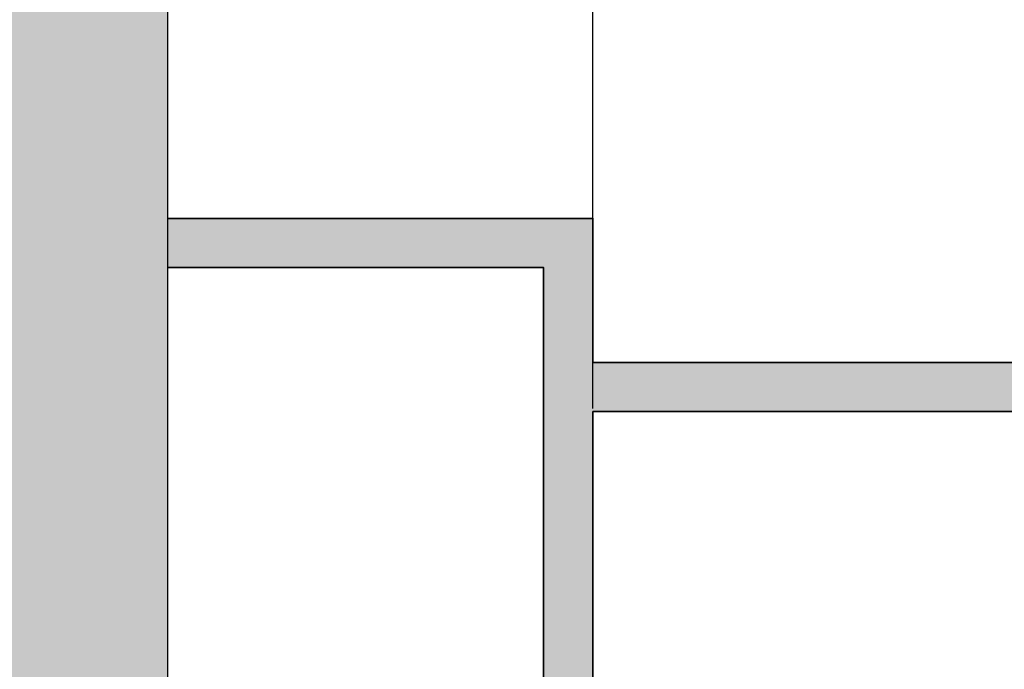
# Model space of a CAD drawing. Units: millimetres. Extents: x -22994 to 29398, y -19990 to 20176.
# Tile 29 of 135: x 99 to 119, y 43 to 56. Entities that reach past the tile are written whole.
import ezdxf

# ---------------------------------------------------------------- set-up
doc = ezdxf.new("R2010")
doc.units = ezdxf.units.MM
doc.header["$MEASUREMENT"] = 0
for name, color, linetype, lineweight in [('M-DIMS', 2, 'Continuous', 18), ('M-EQPM', 7, 'Continuous', 25), ('M-EQPM-PATT', 7, 'Continuous', 18), ('M-PIPE', 7, 'Continuous', 35)]:
    doc.layers.add(name, color=color, linetype=linetype, lineweight=lineweight)
doc.styles.get("Standard").update_dxf_attribs({"font": 'arial.ttf'})
doc.dimstyles.get("Standard").update_dxf_attribs({"dimtxt": 0.18, "dimasz": 10000, "dimexe": 0.18, "dimexo": 0.0625, "dimgap": 0.09, "dimtad": 0, "dimtih": 1, "dimtoh": 1, "dimdec": 0, "dimzin": 0, "dimdsep": 46, "dimtxsty": 'Standard', "dimcen": 0.09, "dimadec": 0, "dimazin": 0, "dimtfac": 1, "dimtdec": 0, "dimtofl": 0, "dimtmove": 0, "dimatfit": 3, "dimfxl": 1, "dimtolj": 1, "dimtzin": 0, "dimlwd": 30, "dimarcsym": 0})

# ---------------------------------------------------------------- blocks, each defined once
blk = doc.blocks.new('*D2')
at = {"layer": 'Defpoints', "color": 0, "transparency": 16777216}
for p in [(6.677, 10.271), (290.852, 10.271), (290.852, -5.079)]:
    blk.add_point(p, dxfattribs=at)
at = {"layer": 'M-DIMS', "color": 0, "lineweight": -2, "transparency": 16777216}
for p, q in [((6.677, 10.209), (6.677, -5.259)), ((290.852, 10.209), (290.852, -5.259))]:
    blk.add_line(p, q, dxfattribs=at)
at = {"layer": 'M-DIMS', "color": 0, "lineweight": 30, "transparency": 16777216}
for p, q in [((-9993.323, -5.079), (-19993.323, -5.079)), ((10290.852, -5.079), (20290.852, -5.079))]:
    blk.add_line(p, q, dxfattribs=at)
at = {"layer": 'M-DIMS', "color": 0, "transparency": 16777216}
for points in [[(-9993.323, 1661.588), (-9993.323, -1671.745), (6.677, -5.079)], [(10290.852, 1661.588), (10290.852, -1671.745), (290.852, -5.079)]]:
    blk.add_solid(points, dxfattribs=at)
at = {"layer": 'M-DIMS', "color": 0, "transparency": 16777216, "insert": (148.765, -5.079), "char_height": 0.18, "attachment_point": 5}
blk.add_mtext('\\A1;284.2', dxfattribs=at)
blk = doc.blocks.new('*D3')
at = {"layer": 'Defpoints', "color": 0, "transparency": 16777216}
for p in [(110.265, 204.165), (110.265, 176.366), (95.833, 127.967)]:
    blk.add_point(p, dxfattribs=at)
at = {"layer": 'M-DIMS', "color": 0, "lineweight": -2, "transparency": 16777216}
for p, q in [((95.833, 128.03), (95.833, 204.345)), ((110.265, 176.429), (110.265, 204.345))]:
    blk.add_line(p, q, dxfattribs=at)
at = {"layer": 'M-DIMS', "color": 0, "lineweight": 30, "transparency": 16777216}
for p, q in [((-9904.167, 204.165), (-19904.167, 204.165)), ((10110.265, 204.165), (20110.265, 204.165))]:
    blk.add_line(p, q, dxfattribs=at)
at = {"layer": 'M-DIMS', "color": 0, "transparency": 16777216}
for points in [[(-9904.167, 1870.832), (-9904.167, -1462.501), (95.833, 204.165)], [(10110.265, 1870.832), (10110.265, -1462.501), (110.265, 204.165)]]:
    blk.add_solid(points, dxfattribs=at)
at = {"layer": 'M-DIMS', "color": 0, "transparency": 16777216, "insert": (103.049, 204.165), "char_height": 0.18, "attachment_point": 5}
blk.add_mtext('\\A1;14.432', dxfattribs=at)
blk = doc.blocks.new('*D4')
at = {"layer": 'Defpoints', "color": 0, "transparency": 16777216}
for p in [(116.265, 204.165), (110.265, 176.366), (116.265, 176.366)]:
    blk.add_point(p, dxfattribs=at)
at = {"layer": 'M-DIMS', "color": 0, "lineweight": -2, "transparency": 16777216}
for p, q in [((110.265, 176.429), (110.265, 204.345)), ((116.265, 176.429), (116.265, 204.345))]:
    blk.add_line(p, q, dxfattribs=at)
at = {"layer": 'M-DIMS', "color": 0, "lineweight": 30, "transparency": 16777216}
for p, q in [((-9889.735, 204.165), (-19889.735, 204.165)), ((10116.265, 204.165), (20116.265, 204.165))]:
    blk.add_line(p, q, dxfattribs=at)
at = {"layer": 'M-DIMS', "color": 0, "transparency": 16777216}
for points in [[(-9889.735, 1870.832), (-9889.735, -1462.501), (110.265, 204.165)], [(10116.265, 1870.832), (10116.265, -1462.501), (116.265, 204.165)]]:
    blk.add_solid(points, dxfattribs=at)
at = {"layer": 'M-DIMS', "color": 0, "transparency": 16777216, "insert": (113.265, 204.165), "char_height": 0.18, "attachment_point": 5}
blk.add_mtext('\\A1;6', dxfattribs=at)
blk = doc.blocks.new('*D5')
at = {"layer": 'Defpoints', "color": 0, "transparency": 16777216}
for p in [(181.265, 204.165), (116.265, 176.366), (181.265, 176.366)]:
    blk.add_point(p, dxfattribs=at)
at = {"layer": 'M-DIMS', "color": 0, "lineweight": -2, "transparency": 16777216}
for p, q in [((116.265, 176.429), (116.265, 204.345)), ((181.265, 176.429), (181.265, 204.345))]:
    blk.add_line(p, q, dxfattribs=at)
at = {"layer": 'M-DIMS', "color": 0, "lineweight": 30, "transparency": 16777216}
for p, q in [((-9883.735, 204.165), (-19883.735, 204.165)), ((10181.265, 204.165), (20181.265, 204.165))]:
    blk.add_line(p, q, dxfattribs=at)
at = {"layer": 'M-DIMS', "color": 0, "transparency": 16777216}
for points in [[(-9883.735, 1870.832), (-9883.735, -1462.501), (116.265, 204.165)], [(10181.265, 1870.832), (10181.265, -1462.501), (181.265, 204.165)]]:
    blk.add_solid(points, dxfattribs=at)
at = {"layer": 'M-DIMS', "color": 0, "transparency": 16777216, "insert": (148.765, 204.165), "char_height": 0.18, "attachment_point": 5}
blk.add_mtext('\\A1;65', dxfattribs=at)
blk = doc.blocks.new('*D6')
at = {"layer": 'Defpoints', "color": 0, "transparency": 16777216}
for p in [(187.265, 204.165), (181.265, 176.366), (187.265, 176.366)]:
    blk.add_point(p, dxfattribs=at)
at = {"layer": 'M-DIMS', "color": 0, "lineweight": -2, "transparency": 16777216}
for p, q in [((181.265, 176.429), (181.265, 204.345)), ((187.265, 176.429), (187.265, 204.345))]:
    blk.add_line(p, q, dxfattribs=at)
at = {"layer": 'M-DIMS', "color": 0, "lineweight": 30, "transparency": 16777216}
for p, q in [((-9818.735, 204.165), (-19818.735, 204.165)), ((10187.265, 204.165), (20187.265, 204.165))]:
    blk.add_line(p, q, dxfattribs=at)
at = {"layer": 'M-DIMS', "color": 0, "transparency": 16777216}
for points in [[(-9818.735, 1870.832), (-9818.735, -1462.501), (181.265, 204.165)], [(10187.265, 1870.832), (10187.265, -1462.501), (187.265, 204.165)]]:
    blk.add_solid(points, dxfattribs=at)
at = {"layer": 'M-DIMS', "color": 0, "transparency": 16777216, "insert": (184.265, 204.165), "char_height": 0.18, "attachment_point": 5}
blk.add_mtext('\\A1;6', dxfattribs=at)
blk = doc.blocks.new('*D7')
at = {"layer": 'Defpoints', "color": 0, "transparency": 16777216}
for p in [(201.697, 204.165), (187.265, 176.366), (201.697, 127.967)]:
    blk.add_point(p, dxfattribs=at)
at = {"layer": 'M-DIMS', "color": 0, "lineweight": -2, "transparency": 16777216}
for p, q in [((187.265, 176.429), (187.265, 204.345)), ((201.697, 128.03), (201.697, 204.345))]:
    blk.add_line(p, q, dxfattribs=at)
at = {"layer": 'M-DIMS', "color": 0, "lineweight": 30, "transparency": 16777216}
for p, q in [((-9812.735, 204.165), (-19812.735, 204.165)), ((10201.697, 204.165), (20201.697, 204.165))]:
    blk.add_line(p, q, dxfattribs=at)
at = {"layer": 'M-DIMS', "color": 0, "transparency": 16777216}
for points in [[(-9812.735, 1870.832), (-9812.735, -1462.501), (187.265, 204.165)], [(10201.697, 1870.832), (10201.697, -1462.501), (201.697, 204.165)]]:
    blk.add_solid(points, dxfattribs=at)
at = {"layer": 'M-DIMS', "color": 0, "transparency": 16777216, "insert": (194.481, 204.165), "char_height": 0.18, "attachment_point": 5}
blk.add_mtext('\\A1;14.432', dxfattribs=at)
blk = doc.blocks.new('*D8')
at = {"layer": 'Defpoints', "color": 0, "transparency": 16777216}
for p in [(227.648, 204.165), (227.648, 146.73), (201.697, 127.967)]:
    blk.add_point(p, dxfattribs=at)
at = {"layer": 'M-DIMS', "color": 0, "lineweight": -2, "transparency": 16777216}
for p, q in [((201.697, 128.03), (201.697, 204.345)), ((227.648, 146.792), (227.648, 204.345))]:
    blk.add_line(p, q, dxfattribs=at)
at = {"layer": 'M-DIMS', "color": 0, "lineweight": 30, "transparency": 16777216}
for p, q in [((-9798.303, 204.165), (-19798.303, 204.165)), ((10227.648, 204.165), (20227.648, 204.165))]:
    blk.add_line(p, q, dxfattribs=at)
at = {"layer": 'M-DIMS', "color": 0, "transparency": 16777216}
for points in [[(-9798.303, 1870.832), (-9798.303, -1462.501), (201.697, 204.165)], [(10227.648, 1870.832), (10227.648, -1462.501), (227.648, 204.165)]]:
    blk.add_solid(points, dxfattribs=at)
at = {"layer": 'M-DIMS', "color": 0, "transparency": 16777216, "insert": (214.673, 204.165), "char_height": 0.18, "attachment_point": 5}
blk.add_mtext('\\A1;25.95', dxfattribs=at)
blk = doc.blocks.new('*D9')
at = {"layer": 'Defpoints', "color": 0, "transparency": 16777216}
for p in [(187.265, 176.366), (306.202, 176.366), (290.852, 10.271)]:
    blk.add_point(p, dxfattribs=at)
at = {"layer": 'M-DIMS', "color": 0, "lineweight": 30, "transparency": 16777216}
for p, q in [((306.202, 10176.366), (306.202, 20176.366)), ((306.202, -9989.729), (306.202, -19989.729))]:
    blk.add_line(p, q, dxfattribs=at)
at = {"layer": 'M-DIMS', "color": 0, "lineweight": -2, "transparency": 16777216}
for p, q in [((187.327, 176.366), (306.382, 176.366)), ((290.915, 10.271), (306.382, 10.271))]:
    blk.add_line(p, q, dxfattribs=at)
at = {"layer": 'M-DIMS', "color": 0, "transparency": 16777216}
for points in [[(-1360.465, 10176.366), (1972.869, 10176.366), (306.202, 176.366)], [(-1360.465, -9989.729), (1972.869, -9989.729), (306.202, 10.271)]]:
    blk.add_solid(points, dxfattribs=at)
at = {"layer": 'M-DIMS', "color": 0, "transparency": 16777216, "insert": (306.202, 93.319), "char_height": 0.18, "attachment_point": 5}
blk.add_mtext('\\A1;166.1', dxfattribs=at)
blk = doc.blocks.new('*D10')
at = {"layer": 'Defpoints', "color": 0, "transparency": 16777216}
for p in [(125.65, 136.071), (133.346, 136.071), (133.346, -5.079)]:
    blk.add_point(p, dxfattribs=at)
at = {"layer": 'M-DIMS', "color": 0, "lineweight": -2, "transparency": 16777216}
for p, q in [((125.65, 136.009), (125.65, -5.259)), ((133.346, 136.009), (133.346, -5.259))]:
    blk.add_line(p, q, dxfattribs=at)
at = {"layer": 'M-DIMS', "color": 0, "lineweight": 30, "transparency": 16777216}
for p, q in [((-9874.35, -5.079), (-19874.35, -5.079)), ((10133.346, -5.079), (20133.346, -5.079))]:
    blk.add_line(p, q, dxfattribs=at)
at = {"layer": 'M-DIMS', "color": 0, "transparency": 16777216}
for points in [[(-9874.35, 1661.588), (-9874.35, -1671.745), (125.65, -5.079)], [(10133.346, 1661.588), (10133.346, -1671.745), (133.346, -5.079)]]:
    blk.add_solid(points, dxfattribs=at)
at = {"layer": 'M-DIMS', "color": 0, "transparency": 16777216, "insert": (129.498, -5.079), "char_height": 0.18, "attachment_point": 5}
blk.add_mtext('\\A1;7.696', dxfattribs=at)
blk = doc.blocks.new('*D11')
at = {"layer": 'Defpoints', "color": 0, "transparency": 16777216}
for p in [(133.346, 136.071), (135.65, 136.071), (135.65, -5.079)]:
    blk.add_point(p, dxfattribs=at)
at = {"layer": 'M-DIMS', "color": 0, "lineweight": -2, "transparency": 16777216}
for p, q in [((133.346, 136.009), (133.346, -5.259)), ((135.65, 136.009), (135.65, -5.259))]:
    blk.add_line(p, q, dxfattribs=at)
at = {"layer": 'M-DIMS', "color": 0, "lineweight": 30, "transparency": 16777216}
for p, q in [((-9866.654, -5.079), (-19866.654, -5.079)), ((10135.65, -5.079), (20135.65, -5.079))]:
    blk.add_line(p, q, dxfattribs=at)
at = {"layer": 'M-DIMS', "color": 0, "transparency": 16777216}
for points in [[(-9866.654, 1661.588), (-9866.654, -1671.745), (133.346, -5.079)], [(10135.65, 1661.588), (10135.65, -1671.745), (135.65, -5.079)]]:
    blk.add_solid(points, dxfattribs=at)
at = {"layer": 'M-DIMS', "color": 0, "transparency": 16777216, "insert": (134.498, -5.079), "char_height": 0.18, "attachment_point": 5}
blk.add_mtext('\\A1;2.304', dxfattribs=at)
blk = doc.blocks.new('*D12')
at = {"layer": 'Defpoints', "color": 0, "transparency": 16777216}
for p in [(135.65, 136.071), (145.65, 136.071), (145.65, -5.079)]:
    blk.add_point(p, dxfattribs=at)
at = {"layer": 'M-DIMS', "color": 0, "lineweight": -2, "transparency": 16777216}
for p, q in [((135.65, 136.009), (135.65, -5.259)), ((145.65, 136.009), (145.65, -5.259))]:
    blk.add_line(p, q, dxfattribs=at)
at = {"layer": 'M-DIMS', "color": 0, "lineweight": 30, "transparency": 16777216}
for p, q in [((-9864.35, -5.079), (-19864.35, -5.079)), ((10145.65, -5.079), (20145.65, -5.079))]:
    blk.add_line(p, q, dxfattribs=at)
at = {"layer": 'M-DIMS', "color": 0, "transparency": 16777216}
for points in [[(-9864.35, 1661.588), (-9864.35, -1671.745), (135.65, -5.079)], [(10145.65, 1661.588), (10145.65, -1671.745), (145.65, -5.079)]]:
    blk.add_solid(points, dxfattribs=at)
at = {"layer": 'M-DIMS', "color": 0, "transparency": 16777216, "insert": (140.65, -5.079), "char_height": 0.18, "attachment_point": 5}
blk.add_mtext('\\A1;10', dxfattribs=at)
blk = doc.blocks.new('*D13')
at = {"layer": 'Defpoints', "color": 0, "transparency": 16777216}
for p in [(145.65, 136.071), (155.65, 136.071), (155.65, -5.079)]:
    blk.add_point(p, dxfattribs=at)
at = {"layer": 'M-DIMS', "color": 0, "lineweight": -2, "transparency": 16777216}
for p, q in [((145.65, 136.009), (145.65, -5.259)), ((155.65, 136.009), (155.65, -5.259))]:
    blk.add_line(p, q, dxfattribs=at)
at = {"layer": 'M-DIMS', "color": 0, "lineweight": 30, "transparency": 16777216}
for p, q in [((-9854.35, -5.079), (-19854.35, -5.079)), ((10155.65, -5.079), (20155.65, -5.079))]:
    blk.add_line(p, q, dxfattribs=at)
at = {"layer": 'M-DIMS', "color": 0, "transparency": 16777216}
for points in [[(-9854.35, 1661.588), (-9854.35, -1671.745), (145.65, -5.079)], [(10155.65, 1661.588), (10155.65, -1671.745), (155.65, -5.079)]]:
    blk.add_solid(points, dxfattribs=at)
at = {"layer": 'M-DIMS', "color": 0, "transparency": 16777216, "insert": (150.65, -5.079), "char_height": 0.18, "attachment_point": 5}
blk.add_mtext('\\A1;10', dxfattribs=at)
blk = doc.blocks.new('*D14')
at = {"layer": 'Defpoints', "color": 0, "transparency": 16777216}
for p in [(155.65, 136.071), (165.65, 136.071), (165.65, -5.079)]:
    blk.add_point(p, dxfattribs=at)
at = {"layer": 'M-DIMS', "color": 0, "lineweight": -2, "transparency": 16777216}
for p, q in [((155.65, 136.009), (155.65, -5.259)), ((165.65, 136.009), (165.65, -5.259))]:
    blk.add_line(p, q, dxfattribs=at)
at = {"layer": 'M-DIMS', "color": 0, "lineweight": 30, "transparency": 16777216}
for p, q in [((-9844.35, -5.079), (-19844.35, -5.079)), ((10165.65, -5.079), (20165.65, -5.079))]:
    blk.add_line(p, q, dxfattribs=at)
at = {"layer": 'M-DIMS', "color": 0, "transparency": 16777216}
for points in [[(-9844.35, 1661.588), (-9844.35, -1671.745), (155.65, -5.079)], [(10165.65, 1661.588), (10165.65, -1671.745), (165.65, -5.079)]]:
    blk.add_solid(points, dxfattribs=at)
at = {"layer": 'M-DIMS', "color": 0, "transparency": 16777216, "insert": (160.65, -5.079), "char_height": 0.18, "attachment_point": 5}
blk.add_mtext('\\A1;10', dxfattribs=at)
blk = doc.blocks.new('*D15')
at = {"layer": 'Defpoints', "color": 0, "transparency": 16777216}
for p in [(173.346, 154.788), (173.346, 136.071), (306.202, 136.071)]:
    blk.add_point(p, dxfattribs=at)
at = {"layer": 'M-DIMS', "color": 0, "lineweight": 30, "transparency": 16777216}
for p, q in [((306.202, 10154.788), (306.202, 20154.788)), ((306.202, -9863.929), (306.202, -19863.929))]:
    blk.add_line(p, q, dxfattribs=at)
at = {"layer": 'M-DIMS', "color": 0, "lineweight": -2, "transparency": 16777216}
for p, q in [((173.408, 154.788), (306.382, 154.788)), ((173.408, 136.071), (306.382, 136.071))]:
    blk.add_line(p, q, dxfattribs=at)
at = {"layer": 'M-DIMS', "color": 0, "transparency": 16777216}
for points in [[(-1360.465, 10154.788), (1972.869, 10154.788), (306.202, 154.788)], [(-1360.465, -9863.929), (1972.869, -9863.929), (306.202, 136.071)]]:
    blk.add_solid(points, dxfattribs=at)
at = {"layer": 'M-DIMS', "color": 0, "transparency": 16777216, "insert": (306.202, 145.43), "char_height": 0.18, "attachment_point": 5}
blk.add_mtext('\\A1;18.717', dxfattribs=at)
blk = doc.blocks.new('*D16')
at = {"layer": 'Defpoints', "color": 0, "transparency": 16777216}
for p in [(120.17, 204.165), (110.466, 48.035), (120.17, 48.035)]:
    blk.add_point(p, dxfattribs=at)
at = {"layer": 'M-DIMS', "color": 0, "lineweight": -2, "transparency": 16777216}
for p, q in [((110.466, 48.097), (110.466, 204.345)), ((120.17, 48.097), (120.17, 204.345))]:
    blk.add_line(p, q, dxfattribs=at)
at = {"layer": 'M-DIMS', "color": 0, "lineweight": 30, "transparency": 16777216}
for p, q in [((-9889.534, 204.165), (-19889.534, 204.165)), ((10120.17, 204.165), (20120.17, 204.165))]:
    blk.add_line(p, q, dxfattribs=at)
at = {"layer": 'M-DIMS', "color": 0, "transparency": 16777216}
for points in [[(-9889.534, 1870.832), (-9889.534, -1462.501), (110.466, 204.165)], [(10120.17, 1870.832), (10120.17, -1462.501), (120.17, 204.165)]]:
    blk.add_solid(points, dxfattribs=at)
at = {"layer": 'M-DIMS', "color": 0, "transparency": 16777216, "insert": (115.318, 204.165), "char_height": 0.18, "attachment_point": 5}
blk.add_mtext('\\A1;9.704', dxfattribs=at)
blk = doc.blocks.new('*D17')
at = {"layer": 'Defpoints', "color": 0, "transparency": 16777216}
for p in [(126.17, 204.165), (120.17, 48.035), (126.17, 48.035)]:
    blk.add_point(p, dxfattribs=at)
at = {"layer": 'M-DIMS', "color": 0, "lineweight": -2, "transparency": 16777216}
for p, q in [((120.17, 48.097), (120.17, 204.345)), ((126.17, 48.097), (126.17, 204.345))]:
    blk.add_line(p, q, dxfattribs=at)
at = {"layer": 'M-DIMS', "color": 0, "lineweight": 30, "transparency": 16777216}
for p, q in [((-9879.83, 204.165), (-19879.83, 204.165)), ((10126.17, 204.165), (20126.17, 204.165))]:
    blk.add_line(p, q, dxfattribs=at)
at = {"layer": 'M-DIMS', "color": 0, "transparency": 16777216}
for points in [[(-9879.83, 1870.832), (-9879.83, -1462.501), (120.17, 204.165)], [(10126.17, 1870.832), (10126.17, -1462.501), (126.17, 204.165)]]:
    blk.add_solid(points, dxfattribs=at)
at = {"layer": 'M-DIMS', "color": 0, "transparency": 16777216, "insert": (123.17, 204.165), "char_height": 0.18, "attachment_point": 5}
blk.add_mtext('\\A1;6', dxfattribs=at)
blk = doc.blocks.new('*D18')
at = {"layer": 'Defpoints', "color": 0, "transparency": 16777216}
for p in [(132.17, 204.165), (126.17, 48.035), (132.17, 48.035)]:
    blk.add_point(p, dxfattribs=at)
at = {"layer": 'M-DIMS', "color": 0, "lineweight": -2, "transparency": 16777216}
for p, q in [((126.17, 48.097), (126.17, 204.345)), ((132.17, 48.097), (132.17, 204.345))]:
    blk.add_line(p, q, dxfattribs=at)
at = {"layer": 'M-DIMS', "color": 0, "lineweight": 30, "transparency": 16777216}
for p, q in [((-9873.83, 204.165), (-19873.83, 204.165)), ((10132.17, 204.165), (20132.17, 204.165))]:
    blk.add_line(p, q, dxfattribs=at)
at = {"layer": 'M-DIMS', "color": 0, "transparency": 16777216}
for points in [[(-9873.83, 1870.832), (-9873.83, -1462.501), (126.17, 204.165)], [(10132.17, 1870.832), (10132.17, -1462.501), (132.17, 204.165)]]:
    blk.add_solid(points, dxfattribs=at)
at = {"layer": 'M-DIMS', "color": 0, "transparency": 16777216, "insert": (129.17, 204.165), "char_height": 0.18, "attachment_point": 5}
blk.add_mtext('\\A1;6', dxfattribs=at)
blk = doc.blocks.new('*D19')
at = {"layer": 'Defpoints', "color": 0, "transparency": 16777216}
for p in [(138.17, 204.165), (132.17, 48.035), (138.17, 48.035)]:
    blk.add_point(p, dxfattribs=at)
at = {"layer": 'M-DIMS', "color": 0, "lineweight": -2, "transparency": 16777216}
for p, q in [((132.17, 48.097), (132.17, 204.345)), ((138.17, 48.097), (138.17, 204.345))]:
    blk.add_line(p, q, dxfattribs=at)
at = {"layer": 'M-DIMS', "color": 0, "lineweight": 30, "transparency": 16777216}
for p, q in [((-9867.83, 204.165), (-19867.83, 204.165)), ((10138.17, 204.165), (20138.17, 204.165))]:
    blk.add_line(p, q, dxfattribs=at)
at = {"layer": 'M-DIMS', "color": 0, "transparency": 16777216}
for points in [[(-9867.83, 1870.832), (-9867.83, -1462.501), (132.17, 204.165)], [(10138.17, 1870.832), (10138.17, -1462.501), (138.17, 204.165)]]:
    blk.add_solid(points, dxfattribs=at)
at = {"layer": 'M-DIMS', "color": 0, "transparency": 16777216, "insert": (135.17, 204.165), "char_height": 0.18, "attachment_point": 5}
blk.add_mtext('\\A1;6', dxfattribs=at)
blk = doc.blocks.new('*D20')
at = {"layer": 'Defpoints', "color": 0, "transparency": 16777216}
for p in [(144.17, 204.165), (138.17, 48.035), (144.17, 48.035)]:
    blk.add_point(p, dxfattribs=at)
at = {"layer": 'M-DIMS', "color": 0, "lineweight": -2, "transparency": 16777216}
for p, q in [((138.17, 48.097), (138.17, 204.345)), ((144.17, 48.097), (144.17, 204.345))]:
    blk.add_line(p, q, dxfattribs=at)
at = {"layer": 'M-DIMS', "color": 0, "lineweight": 30, "transparency": 16777216}
for p, q in [((-9861.83, 204.165), (-19861.83, 204.165)), ((10144.17, 204.165), (20144.17, 204.165))]:
    blk.add_line(p, q, dxfattribs=at)
at = {"layer": 'M-DIMS', "color": 0, "transparency": 16777216}
for points in [[(-9861.83, 1870.832), (-9861.83, -1462.501), (138.17, 204.165)], [(10144.17, 1870.832), (10144.17, -1462.501), (144.17, 204.165)]]:
    blk.add_solid(points, dxfattribs=at)
at = {"layer": 'M-DIMS', "color": 0, "transparency": 16777216, "insert": (141.17, 204.165), "char_height": 0.18, "attachment_point": 5}
blk.add_mtext('\\A1;6', dxfattribs=at)
blk = doc.blocks.new('*D21')
at = {"layer": 'Defpoints', "color": 0, "transparency": 16777216}
for p in [(149.116, 204.165), (144.17, 48.035), (149.116, 48.035)]:
    blk.add_point(p, dxfattribs=at)
at = {"layer": 'M-DIMS', "color": 0, "lineweight": -2, "transparency": 16777216}
for p, q in [((144.17, 48.097), (144.17, 204.345)), ((149.116, 48.097), (149.116, 204.345))]:
    blk.add_line(p, q, dxfattribs=at)
at = {"layer": 'M-DIMS', "color": 0, "lineweight": 30, "transparency": 16777216}
for p, q in [((-9855.83, 204.165), (-19855.83, 204.165)), ((10149.116, 204.165), (20149.116, 204.165))]:
    blk.add_line(p, q, dxfattribs=at)
at = {"layer": 'M-DIMS', "color": 0, "transparency": 16777216}
for points in [[(-9855.83, 1870.832), (-9855.83, -1462.501), (144.17, 204.165)], [(10149.116, 1870.832), (10149.116, -1462.501), (149.116, 204.165)]]:
    blk.add_solid(points, dxfattribs=at)
at = {"layer": 'M-DIMS', "color": 0, "transparency": 16777216, "insert": (146.643, 204.165), "char_height": 0.18, "attachment_point": 5}
blk.add_mtext('\\A1;4.945', dxfattribs=at)
blk = doc.blocks.new('*D22')
at = {"layer": 'Defpoints', "color": 0, "transparency": 16777216}
for p in [(149.116, 30.99), (155.116, 30.99), (155.116, -5.079)]:
    blk.add_point(p, dxfattribs=at)
at = {"layer": 'M-DIMS', "color": 0, "lineweight": -2, "transparency": 16777216}
for p, q in [((149.116, 30.927), (149.116, -5.259)), ((155.116, 30.927), (155.116, -5.259))]:
    blk.add_line(p, q, dxfattribs=at)
at = {"layer": 'M-DIMS', "color": 0, "lineweight": 30, "transparency": 16777216}
for p, q in [((-9850.884, -5.079), (-19850.884, -5.079)), ((10155.116, -5.079), (20155.116, -5.079))]:
    blk.add_line(p, q, dxfattribs=at)
at = {"layer": 'M-DIMS', "color": 0, "transparency": 16777216}
for points in [[(-9850.884, 1661.588), (-9850.884, -1671.745), (149.116, -5.079)], [(10155.116, 1661.588), (10155.116, -1671.745), (155.116, -5.079)]]:
    blk.add_solid(points, dxfattribs=at)
at = {"layer": 'M-DIMS', "color": 0, "transparency": 16777216, "insert": (152.116, -5.079), "char_height": 0.18, "attachment_point": 5}
blk.add_mtext('\\A1;6', dxfattribs=at)
blk = doc.blocks.new('*D23')
at = {"layer": 'Defpoints', "color": 0, "transparency": 16777216}
for p in [(155.116, 30.99), (161.116, 30.99), (161.116, -5.079)]:
    blk.add_point(p, dxfattribs=at)
at = {"layer": 'M-DIMS', "color": 0, "lineweight": -2, "transparency": 16777216}
for p, q in [((155.116, 30.927), (155.116, -5.259)), ((161.116, 30.927), (161.116, -5.259))]:
    blk.add_line(p, q, dxfattribs=at)
at = {"layer": 'M-DIMS', "color": 0, "lineweight": 30, "transparency": 16777216}
for p, q in [((-9844.884, -5.079), (-19844.884, -5.079)), ((10161.116, -5.079), (20161.116, -5.079))]:
    blk.add_line(p, q, dxfattribs=at)
at = {"layer": 'M-DIMS', "color": 0, "transparency": 16777216}
for points in [[(-9844.884, 1661.588), (-9844.884, -1671.745), (155.116, -5.079)], [(10161.116, 1661.588), (10161.116, -1671.745), (161.116, -5.079)]]:
    blk.add_solid(points, dxfattribs=at)
at = {"layer": 'M-DIMS', "color": 0, "transparency": 16777216, "insert": (158.116, -5.079), "char_height": 0.18, "attachment_point": 5}
blk.add_mtext('\\A1;6', dxfattribs=at)
blk = doc.blocks.new('*D24')
at = {"layer": 'Defpoints', "color": 0, "transparency": 16777216}
for p in [(161.116, 30.99), (166.439, 30.99), (166.439, -5.079)]:
    blk.add_point(p, dxfattribs=at)
at = {"layer": 'M-DIMS', "color": 0, "lineweight": -2, "transparency": 16777216}
for p, q in [((161.116, 30.927), (161.116, -5.259)), ((166.439, 30.927), (166.439, -5.259))]:
    blk.add_line(p, q, dxfattribs=at)
at = {"layer": 'M-DIMS', "color": 0, "lineweight": 30, "transparency": 16777216}
for p, q in [((-9838.884, -5.079), (-19838.884, -5.079)), ((10166.439, -5.079), (20166.439, -5.079))]:
    blk.add_line(p, q, dxfattribs=at)
at = {"layer": 'M-DIMS', "color": 0, "transparency": 16777216}
for points in [[(-9838.884, 1661.588), (-9838.884, -1671.745), (161.116, -5.079)], [(10166.439, 1661.588), (10166.439, -1671.745), (166.439, -5.079)]]:
    blk.add_solid(points, dxfattribs=at)
at = {"layer": 'M-DIMS', "color": 0, "transparency": 16777216, "insert": (163.777, -5.079), "char_height": 0.18, "attachment_point": 5}
blk.add_mtext('\\A1;5.323', dxfattribs=at)
blk = doc.blocks.new('*D25')
at = {"layer": 'Defpoints', "color": 0, "transparency": 16777216}
for p in [(166.439, 30.99), (172.439, 30.99), (172.439, -5.079)]:
    blk.add_point(p, dxfattribs=at)
at = {"layer": 'M-DIMS', "color": 0, "lineweight": -2, "transparency": 16777216}
for p, q in [((166.439, 30.927), (166.439, -5.259)), ((172.439, 30.927), (172.439, -5.259))]:
    blk.add_line(p, q, dxfattribs=at)
at = {"layer": 'M-DIMS', "color": 0, "lineweight": 30, "transparency": 16777216}
for p, q in [((-9833.561, -5.079), (-19833.561, -5.079)), ((10172.439, -5.079), (20172.439, -5.079))]:
    blk.add_line(p, q, dxfattribs=at)
at = {"layer": 'M-DIMS', "color": 0, "transparency": 16777216}
for points in [[(-9833.561, 1661.588), (-9833.561, -1671.745), (166.439, -5.079)], [(10172.439, 1661.588), (10172.439, -1671.745), (172.439, -5.079)]]:
    blk.add_solid(points, dxfattribs=at)
at = {"layer": 'M-DIMS', "color": 0, "transparency": 16777216, "insert": (169.439, -5.079), "char_height": 0.18, "attachment_point": 5}
blk.add_mtext('\\A1;6', dxfattribs=at)
blk = doc.blocks.new('*D26')
at = {"layer": 'Defpoints', "color": 0, "transparency": 16777216}
for p in [(172.439, 30.99), (178.439, 30.99), (178.439, -5.079)]:
    blk.add_point(p, dxfattribs=at)
at = {"layer": 'M-DIMS', "color": 0, "lineweight": -2, "transparency": 16777216}
for p, q in [((172.439, 30.927), (172.439, -5.259)), ((178.439, 30.927), (178.439, -5.259))]:
    blk.add_line(p, q, dxfattribs=at)
at = {"layer": 'M-DIMS', "color": 0, "lineweight": 30, "transparency": 16777216}
for p, q in [((-9827.561, -5.079), (-19827.561, -5.079)), ((10178.439, -5.079), (20178.439, -5.079))]:
    blk.add_line(p, q, dxfattribs=at)
at = {"layer": 'M-DIMS', "color": 0, "transparency": 16777216}
for points in [[(-9827.561, 1661.588), (-9827.561, -1671.745), (172.439, -5.079)], [(10178.439, 1661.588), (10178.439, -1671.745), (178.439, -5.079)]]:
    blk.add_solid(points, dxfattribs=at)
at = {"layer": 'M-DIMS', "color": 0, "transparency": 16777216, "insert": (175.439, -5.079), "char_height": 0.18, "attachment_point": 5}
blk.add_mtext('\\A1;6', dxfattribs=at)
blk = doc.blocks.new('*D27')
at = {"layer": 'Defpoints', "color": 0, "transparency": 16777216}
for p in [(178.439, 30.99), (188.117, 30.99), (188.117, -5.079)]:
    blk.add_point(p, dxfattribs=at)
at = {"layer": 'M-DIMS', "color": 0, "lineweight": -2, "transparency": 16777216}
for p, q in [((178.439, 30.927), (178.439, -5.259)), ((188.117, 30.927), (188.117, -5.259))]:
    blk.add_line(p, q, dxfattribs=at)
at = {"layer": 'M-DIMS', "color": 0, "lineweight": 30, "transparency": 16777216}
for p, q in [((-9821.561, -5.079), (-19821.561, -5.079)), ((10188.117, -5.079), (20188.117, -5.079))]:
    blk.add_line(p, q, dxfattribs=at)
at = {"layer": 'M-DIMS', "color": 0, "transparency": 16777216}
for points in [[(-9821.561, 1661.588), (-9821.561, -1671.745), (178.439, -5.079)], [(10188.117, 1661.588), (10188.117, -1671.745), (188.117, -5.079)]]:
    blk.add_solid(points, dxfattribs=at)
at = {"layer": 'M-DIMS', "color": 0, "transparency": 16777216, "insert": (183.278, -5.079), "char_height": 0.18, "attachment_point": 5}
blk.add_mtext('\\A1;9.679', dxfattribs=at)
blk = doc.blocks.new('*D28')
at = {"layer": 'Defpoints', "color": 0, "transparency": 16777216}
for p in [(188.117, 48.035), (306.202, 48.035), (188.117, 30.99)]:
    blk.add_point(p, dxfattribs=at)
at = {"layer": 'M-DIMS', "color": 0, "lineweight": 30, "transparency": 16777216}
for p, q in [((306.202, 10048.035), (306.202, 20048.035)), ((306.202, -9969.01), (306.202, -19969.01))]:
    blk.add_line(p, q, dxfattribs=at)
at = {"layer": 'M-DIMS', "color": 0, "lineweight": -2, "transparency": 16777216}
for p, q in [((188.18, 48.035), (306.382, 48.035)), ((188.18, 30.99), (306.382, 30.99))]:
    blk.add_line(p, q, dxfattribs=at)
at = {"layer": 'M-DIMS', "color": 0, "transparency": 16777216}
for points in [[(-1360.465, 10048.035), (1972.869, 10048.035), (306.202, 48.035)], [(-1360.465, -9969.01), (1972.869, -9969.01), (306.202, 30.99)]]:
    blk.add_solid(points, dxfattribs=at)
at = {"layer": 'M-DIMS', "color": 0, "transparency": 16777216, "insert": (306.202, 39.512), "char_height": 0.18, "attachment_point": 5}
blk.add_mtext('\\A1;17.045', dxfattribs=at)
blk = doc.blocks.new('*D29')
at = {"layer": 'Defpoints', "color": 0, "transparency": 16777216}
for p in [(36.801, 80.045), (64.03, 80.045)]:
    blk.add_point(p, dxfattribs=at)
at = {"layer": 'M-DIMS', "color": 0, "lineweight": -2, "transparency": 16777216}
for p, q in [((50.415, 79.955), (50.415, 80.135)), ((50.325, 80.045), (50.505, 80.045))]:
    blk.add_line(p, q, dxfattribs=at)
at = {"layer": 'M-DIMS', "color": 0, "lineweight": 30, "transparency": 16777216}
blk.add_line((20064.03, 80.03), (10064.03, 80.038), dxfattribs=at)
at = {"layer": 'M-DIMS', "color": 0, "transparency": 16777216}
blk.add_solid([(10064.031, 1746.704), (10064.028, -1586.629), (64.03, 80.045)], dxfattribs=at)
at = {"layer": 'M-DIMS', "color": 0, "transparency": 16777216, "insert": (20064.521, 80.03), "char_height": 0.18, "attachment_point": 5}
blk.add_mtext('\\A1;∅27.23', dxfattribs=at)
blk = doc.blocks.new('*D36')
at = {"layer": 'Defpoints', "color": 0, "transparency": 16777216}
for p in [(46.39, 31.303), (46.387, 26.593)]:
    blk.add_point(p, dxfattribs=at)
at = {"layer": 'M-DIMS', "color": 0, "lineweight": 30, "transparency": 16777216}
for p, q in [((57.15, 20031.301), (51.77, 10031.302)), ((10057.15, 20031.301), (57.15, 20031.301))]:
    blk.add_line(p, q, dxfattribs=at)
at = {"layer": 'M-DIMS', "color": 0, "lineweight": -2, "transparency": 16777216}
for p, q in [((46.389, 28.858), (46.389, 29.038)), ((46.299, 28.948), (46.479, 28.948))]:
    blk.add_line(p, q, dxfattribs=at)
at = {"layer": 'M-DIMS', "color": 0, "transparency": 16777216}
blk.add_solid([(-1614.896, 10032.199), (1718.436, 10030.405), (46.39, 31.303)], dxfattribs=at)
at = {"layer": 'M-DIMS', "color": 0, "transparency": 16777216, "insert": (10057.554, 20031.301), "char_height": 0.18, "attachment_point": 5}
blk.add_mtext('\\A1;∅4.71', dxfattribs=at)
blk = doc.blocks.new('*D37')
at = {"layer": 'Defpoints', "color": 0, "transparency": 16777216}
for p in [(54.834, 118.615), (59.494, 118.614)]:
    blk.add_point(p, dxfattribs=at)
at = {"layer": 'M-DIMS', "color": 0, "lineweight": -2, "transparency": 16777216}
for p, q in [((57.164, 118.524), (57.164, 118.704)), ((57.074, 118.614), (57.254, 118.614))]:
    blk.add_line(p, q, dxfattribs=at)
at = {"layer": 'M-DIMS', "color": 0, "lineweight": 30, "transparency": 16777216}
blk.add_line((20059.493, 116.253), (10059.494, 117.434), dxfattribs=at)
at = {"layer": 'M-DIMS', "color": 0, "transparency": 16777216}
blk.add_solid([(10059.69, 1784.1), (10059.297, -1549.233), (59.494, 118.614)], dxfattribs=at)
at = {"layer": 'M-DIMS', "color": 0, "transparency": 16777216, "insert": (20059.985, 116.253), "char_height": 0.18, "attachment_point": 5}
blk.add_mtext('\\A1;∅4.659', dxfattribs=at)

msp = doc.modelspace()

# ---------------------------------------------------------------- hatches: boundary and pattern name
at = {"layer": 'M-EQPM-PATT'}
h = msp.add_hatch(color=256, dxfattribs=at)
h.set_gradient(color1=(205, 32, 39), color2=(205, 32, 39), tint=1)
h.paths.add_polyline_path([(116.2647, 150.3662), (116.2647, 170.3662), (116.2647, 176.3662), (110.2647, 176.3662), (110.2647, 152.0276), (95.8327, 127.967), (95.8327, 16.6063), (201.6967, 16.6063), (201.6967, 127.967), (187.2647, 152.0276), (187.2647, 176.3662), (181.2647, 176.3662), (181.2647, 170.3662), (181.2647, 150.3662), (195.6967, 126.3055), (195.6967, 22.6063), (101.8327, 22.6063), (101.8327, 126.3055)])
h.paths.add_polyline_path([(185.2208, 88.6347), (101.8327, 88.6347), (101.8327, 87.6347), (182.8066, 87.6347), (178.7313, 83.5594), (195.6967, 83.5594), (195.6967, 84.5594), (181.1455, 84.5594)], flags=17)
h.paths.add_polyline_path([(95.8327, 88.6347), (60.9779, 88.6347, -0.0228552), (61.7178, 87.6347), (95.8327, 87.6347)])
h.paths.add_polyline_path([(215.6212, 86.5189), (215.6212, 80.5999), (220.5095, 83.5594)])
h.paths.add_polyline_path([(215.6212, 84.5594), (201.6967, 84.5594), (201.6967, 83.5594), (215.6212, 83.5594)])
h.paths.add_polyline_path([(225.3978, 86.5189), (220.5095, 83.5594), (225.3978, 80.5999)])
h.paths.add_polyline_path([(231.6256, 84.5594), (225.3978, 84.5594), (225.3978, 83.5594), (231.6256, 83.5594)])
h = msp.add_hatch(color=256, dxfattribs=at)
h.set_gradient(color1=(19, 155, 72), color2=(88, 186, 72), tint=1, name='CYLINDER')
h.paths.add_polyline_path([(109.4658, 29.9895), (189.1175, 29.9895), (189.1175, 77.6953), (128.1172, 77.6953, 0.4142136), (126.1172, 75.6953), (126.1172, 73.6953, 0.4142136), (128.1172, 71.6953), (178.5136, 71.6953, -0.4142136), (179.5136, 70.6953), (179.5136, 68.6953, -0.4142136), (178.5136, 67.6953), (128.1172, 67.6953, 0.4142136), (126.1172, 65.6953), (126.1172, 63.6953, 0.4142136), (128.1172, 61.6953), (178.5136, 61.6953, -0.4142136), (179.5136, 60.6953), (179.5136, 58.6953, -0.4142136), (178.5136, 57.6953), (109.7466, 57.6953, -0.4142136), (108.7466, 58.6953), (108.7466, 75.5922, 0.4142136), (106.7466, 77.5922), (101.8327, 77.5922), (101.8327, 76.5922), (106.7466, 76.5922, -0.4142136), (107.7466, 75.5922), (107.7466, 58.6953, 0.4142136), (109.7466, 56.6953), (178.5136, 56.6953, 0.4142136), (180.5136, 58.6953), (180.5136, 60.6953, 0.4142136), (178.5136, 62.6953), (128.1172, 62.6953, -0.4142136), (127.1172, 63.6953), (127.1172, 65.6953, -0.4142136), (128.1172, 66.6953), (178.5136, 66.6953, 0.4142136), (180.5136, 68.6953), (180.5136, 70.6953, 0.4142136), (178.5136, 72.6953), (128.1172, 72.6953, -0.4142136), (127.1172, 73.6953), (127.1172, 75.6953, -0.4142136), (128.1172, 76.6953), (188.1175, 76.6953), (188.1175, 49.0349), (110.4658, 49.0349), (110.4658, 51.9576), (101.8327, 51.9576), (101.8327, 50.9576), (109.4658, 50.9576), (109.4658, 48.5349)])
h.paths.add_polyline_path([(110.4658, 48.0349), (188.1175, 48.0349), (188.1175, 30.9895), (110.4658, 30.9895)], flags=16)
h.paths.add_polyline_path([(136.1519, 78.0082), (161.2406, 78.0082), (161.2406, 84.1903), (136.1519, 84.1903)], flags=9)

# ---------------------------------------------------------------- linework, layer by layer
at = {"layer": 'M-EQPM'}
msp.add_lwpolyline([(116.2647, 170.3662), (116.2647, 150.3662), (101.8327, 126.3055), (101.8327, 22.6063), (195.6967, 22.6063), (195.6967, 126.3055), (181.2647, 150.3662), (181.2647, 170.3662)], dxfattribs=at)
at = {"layer": 'M-PIPE'}
for points in [[(110.4658, 49.0349), (110.4658, 51.9576), (101.8327, 51.9576)], [(109.4658, 48.5349), (109.4658, 50.9576), (101.8327, 50.9576)], [(189.1175, 29.9895), (109.4658, 29.9895), (109.4658, 49.0349)], [(110.4658, 49.0349), (188.1175, 49.0349)], [(188.1175, 30.9895), (110.4658, 30.9895), (110.4658, 48.0349), (188.1175, 48.0349)]]:
    msp.add_lwpolyline(points, dxfattribs=at)

# ---------------------------------------------------------------- dimensions: what is measured, and where the dimension line sits
at = {"layer": 'M-DIMS'}
for base, p1, p2, override, picture, middle in [((306.202, 176.3662), (290.852, 10.2713), (187.2647, 176.3662), {"dimdec": 1, "dimlfac": 1, "dimrnd": 0, "dimzin": 0, "dimdsep": 46, "dimlunit": 2}, '*D9', (306.202, 93.3187)), ((306.202, 136.0713), (173.3459, 154.788), (173.3459, 136.0713), {"dimdec": 3, "dimlfac": 1, "dimrnd": 0, "dimzin": 0, "dimdsep": 46, "dimlunit": 2}, '*D15', (306.202, 145.4297)), ((306.202, 48.0349), (188.1175, 30.9895), (188.1175, 48.0349), {"dimdec": 3, "dimlfac": 1, "dimrnd": 0, "dimzin": 0, "dimdsep": 46, "dimlunit": 2}, '*D28', (306.202, 39.5122))]:
    dim = msp.add_linear_dim(base=base, p1=p1, p2=p2, angle=90, dimstyle='Standard', override=override, dxfattribs=at)
    dim.commit()
    dim.dimension.update_dxf_attribs({"geometry": picture, "text_midpoint": middle})
dim = msp.add_diameter_dim_2p(p1=(46.3875, 26.5934), p2=(46.39, 31.3035), dimstyle='Standard', override={"dimdec": 2, "dimlfac": 1, "dimrnd": 0, "dimzin": 0, "dimdsep": 46, "dimlunit": 2}, dxfattribs=at)
dim.commit()
dim.dimension.update_dxf_attribs({"geometry": '*D36', "text_midpoint": (10057.5542, 20031.3006), "dimtype": 163})
for base, p1, p2, override, picture, middle in [((110.2647, 204.1654), (95.8327, 127.967), (110.2647, 176.3662), {"dimdec": 3, "dimlfac": 1, "dimrnd": 0, "dimzin": 0, "dimdsep": 46, "dimlunit": 2}, '*D3', (103.0487, 204.1654)), ((116.2647, 204.1654), (110.2647, 176.3662), (116.2647, 176.3662), {"dimdec": 0, "dimlfac": 1, "dimrnd": 0, "dimzin": 0, "dimdsep": 46, "dimlunit": 2}, '*D4', (113.2647, 204.1654)), ((120.1702, 204.1654), (110.4658, 48.0349), (120.1702, 48.0349), {"dimdec": 3, "dimlfac": 1, "dimrnd": 0, "dimzin": 0, "dimdsep": 46, "dimlunit": 2}, '*D16', (115.318, 204.1654)), ((181.2647, 204.1654), (116.2647, 176.3662), (181.2647, 176.3662), {"dimdec": 0, "dimlfac": 1, "dimrnd": 0, "dimzin": 0, "dimdsep": 46, "dimlunit": 2}, '*D5', (148.7647, 204.1654)), ((126.1702, 204.1654), (120.1702, 48.0349), (126.1702, 48.0349), {"dimdec": 0, "dimlfac": 1, "dimrnd": 0, "dimzin": 0, "dimdsep": 46, "dimlunit": 2}, '*D17', (123.1702, 204.1654)), ((132.1702, 204.1654), (126.1702, 48.0349), (132.1702, 48.0349), {"dimdec": 0, "dimlfac": 1, "dimrnd": 0, "dimzin": 0, "dimdsep": 46, "dimlunit": 2}, '*D18', (129.1702, 204.1654)), ((138.1702, 204.1654), (132.1702, 48.0349), (138.1702, 48.0349), {"dimdec": 0, "dimlfac": 1, "dimrnd": 0, "dimzin": 0, "dimdsep": 46, "dimlunit": 2}, '*D19', (135.1702, 204.1654)), ((144.1702, 204.1654), (138.1702, 48.0349), (144.1702, 48.0349), {"dimdec": 0, "dimlfac": 1, "dimrnd": 0, "dimzin": 0, "dimdsep": 46, "dimlunit": 2}, '*D20', (141.1702, 204.1654)), ((149.11567, 204.16539), (144.17023, 48.03494), (149.11567, 48.03494), {"dimdec": 3, "dimlfac": 1, "dimrnd": 0, "dimzin": 0, "dimdsep": 46, "dimlunit": 2}, '*D21', (146.64295, 204.16539)), ((187.2647, 204.1654), (181.2647, 176.3662), (187.2647, 176.3662), {"dimdec": 0, "dimlfac": 1, "dimrnd": 0, "dimzin": 0, "dimdsep": 46, "dimlunit": 2}, '*D6', (184.2647, 204.1654)), ((201.6967, 204.1654), (187.2647, 176.3662), (201.6967, 127.967), {"dimdec": 3, "dimlfac": 1, "dimrnd": 0, "dimzin": 0, "dimdsep": 46, "dimlunit": 2}, '*D7', (194.4807, 204.1654)), ((227.6485, 204.1654), (201.6967, 127.967), (227.6485, 146.7296), {"dimdec": 2, "dimlfac": 1, "dimrnd": 0, "dimzin": 0, "dimdsep": 46, "dimlunit": 2}, '*D8', (214.6726, 204.1654)), ((290.852, -5.0787), (6.6773, 10.2713), (290.852, 10.2713), {"dimdec": 1, "dimlfac": 1, "dimrnd": 0, "dimzin": 0, "dimdsep": 46, "dimlunit": 2}, '*D2', (148.7647, -5.0787)), ((133.3459, -5.0787), (125.6498, 136.0713), (133.3459, 136.0713), {"dimdec": 3, "dimlfac": 1, "dimrnd": 0, "dimzin": 0, "dimdsep": 46, "dimlunit": 2}, '*D10', (129.4978, -5.0787)), ((135.6498, -5.0787), (133.3459, 136.0713), (135.6498, 136.0713), {"dimdec": 3, "dimlfac": 1, "dimrnd": 0, "dimzin": 0, "dimdsep": 46, "dimlunit": 2}, '*D11', (134.4978, -5.0787)), ((145.6498, -5.0787), (135.6498, 136.0713), (145.6498, 136.0713), {"dimdec": 0, "dimlfac": 1, "dimrnd": 0, "dimzin": 0, "dimdsep": 46, "dimlunit": 2}, '*D12', (140.6498, -5.0787)), ((155.6498, -5.0787), (145.6498, 136.0713), (155.6498, 136.0713), {"dimdec": 0, "dimlfac": 1, "dimrnd": 0, "dimzin": 0, "dimdsep": 46, "dimlunit": 2}, '*D13', (150.6498, -5.0787)), ((155.1157, -5.0787), (149.1157, 30.9895), (155.1157, 30.9895), {"dimdec": 0, "dimlfac": 1, "dimrnd": 0, "dimzin": 0, "dimdsep": 46, "dimlunit": 2}, '*D22', (152.1157, -5.0787)), ((161.1157, -5.0787), (155.1157, 30.9895), (161.1157, 30.9895), {"dimdec": 0, "dimlfac": 1, "dimrnd": 0, "dimzin": 0, "dimdsep": 46, "dimlunit": 2}, '*D23', (158.1157, -5.0787)), ((165.6498, -5.0787), (155.6498, 136.0713), (165.6498, 136.0713), {"dimdec": 0, "dimlfac": 1, "dimrnd": 0, "dimzin": 0, "dimdsep": 46, "dimlunit": 2}, '*D14', (160.6498, -5.0787)), ((166.4387, -5.0787), (161.1157, 30.9895), (166.4387, 30.9895), {"dimdec": 3, "dimlfac": 1, "dimrnd": 0, "dimzin": 0, "dimdsep": 46, "dimlunit": 2}, '*D24', (163.7772, -5.0787)), ((172.4387, -5.0787), (166.4387, 30.9895), (172.4387, 30.9895), {"dimdec": 0, "dimlfac": 1, "dimrnd": 0, "dimzin": 0, "dimdsep": 46, "dimlunit": 2}, '*D25', (169.4387, -5.0787)), ((178.4387, -5.0787), (172.4387, 30.9895), (178.4387, 30.9895), {"dimdec": 0, "dimlfac": 1, "dimrnd": 0, "dimzin": 0, "dimdsep": 46, "dimlunit": 2}, '*D26', (175.4387, -5.0787)), ((188.1175, -5.0787), (178.4387, 30.9895), (188.1175, 30.9895), {"dimdec": 3, "dimlfac": 1, "dimrnd": 0, "dimzin": 0, "dimdsep": 46, "dimlunit": 2}, '*D27', (183.2781, -5.0787))]:
    dim = msp.add_linear_dim(base=base, p1=p1, p2=p2, dimstyle='Standard', override=override, dxfattribs=at)
    dim.commit()
    dim.dimension.update_dxf_attribs({"geometry": picture, "text_midpoint": middle})
for p1, p2, override, picture, middle in [((54.8343, 118.6145), (59.4936, 118.614), {"dimdec": 3, "dimlfac": 1, "dimrnd": 0, "dimzin": 0, "dimdsep": 46, "dimlunit": 2}, '*D37', (20059.4934, 116.2531)), ((36.8006, 80.045), (64.0296, 80.045), {"dimdec": 2, "dimlfac": 1, "dimrnd": 0, "dimzin": 0, "dimdsep": 46, "dimlunit": 2}, '*D29', (20064.0296, 80.0303))]:
    dim = msp.add_diameter_dim_2p(p1=p1, p2=p2, dimstyle='Standard', override=override, dxfattribs=at)
    dim.commit()
    dim.dimension.update_dxf_attribs({"geometry": picture, "text_midpoint": middle})

doc.saveas('drawing.dxf')
